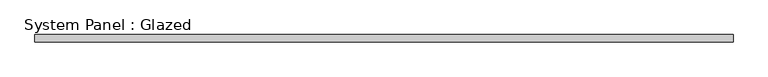
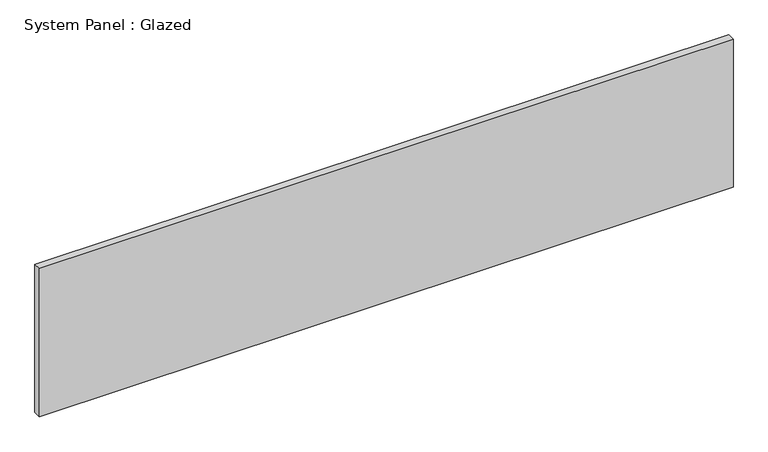
"""IFC4 building model written with IfcOpenShell, lengths in millimetres: plate geometry, System Panel : Glazed."""

from ifc_helpers import new_model, si_unit, origin, origin_with_axes, place, context, project, spatial, polyline, outline, extrude, source, transform, mapped, element, save


def system_panel_glazed_c682d145(model_context):
    return source(origin(), model_context, "Body", "SweptSolid", [
        extrude(outline(polyline([(1171.575, 19.05), (-1171.575, 19.05), (-1171.575, 44.45), (1171.575, 44.45), (1171.575, 19.05)])), origin_with_axes(), (0.0, 0.0, 1.0), 529.155826),
    ])


if __name__ == "__main__":
    model = new_model("IFC4")
    model_context = context("Model", 3, world=origin())
    ifc_project = project(units=[si_unit("LENGTHUNIT", "METRE", prefix="MILLI")], contexts=[model_context])
    site = spatial("IfcSite", under=ifc_project)
    building = spatial("IfcBuilding", under=site)
    placement = place(None, origin())
    system_panel_glazed_shape = system_panel_glazed_c682d145(model_context)
    element("IfcPlate", 1, ObjectType="System Panel : Glazed", at=placement, inside=building, context=model_context, shape_type="MappedRepresentation", body=[
        mapped(system_panel_glazed_shape, transform((0.0, 0.0, 0.0), x_axis=(1.0, 0.0, 0.0), y_axis=(0.0, 1.0, 0.0), z_axis=(0.0, 0.0, 1.0))),
    ])
    save(model, "model.ifc")

# Revit data of these elements
# Type "System Panel : Glazed"
#   Construction Type Id = "GSP4R"
#   Analytic Construction = "1/8 in Pilkington single glazing"
#   Visual Light Transmittance = 0.9
#   Solar Heat Gain Coefficient = 0.86
#   Heat Transfer Coefficient (U) = 1.18115 BTU/(h·ft²·°F)
#   Define Thermal Properties by = 1
# Element 1 (IfcPlate, "System Panel : Glazed")
#   Materials on its faces: "Glass"
# Materials
#   "Glass": class "Glass", colour RGB 0 128 192, transparency 0.75, Description = "Soda Lime Glass", Cost = 0
